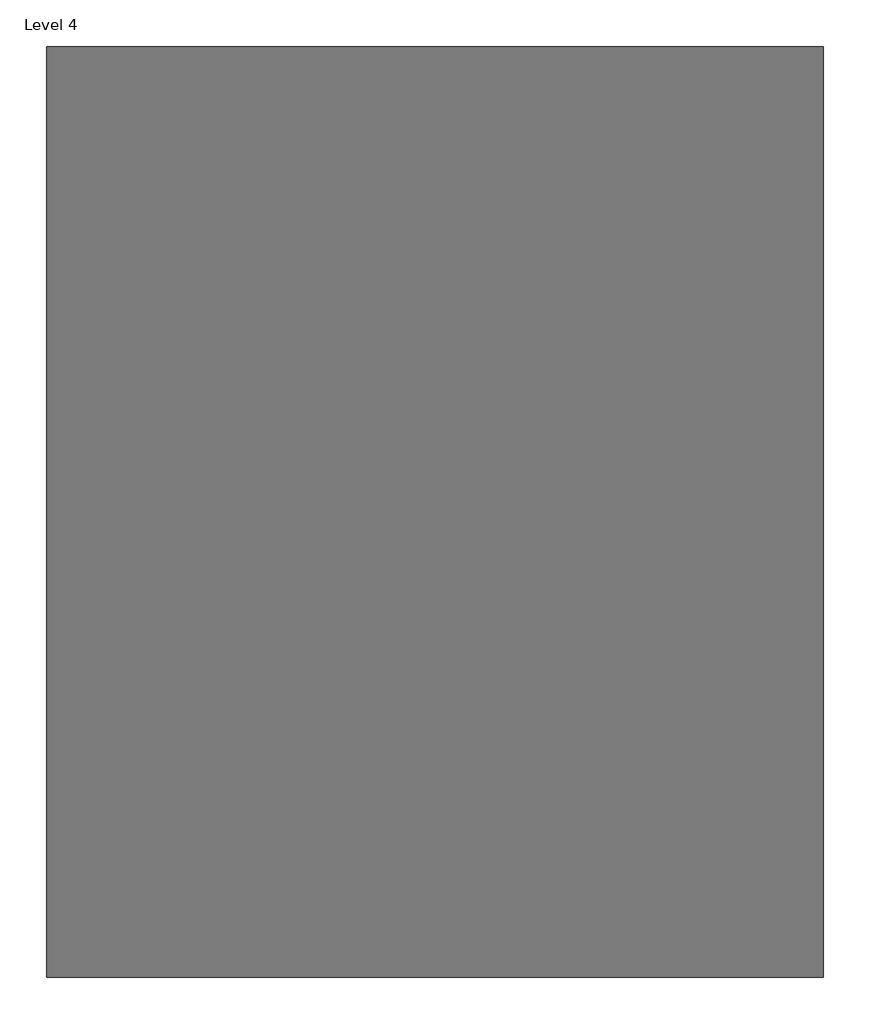
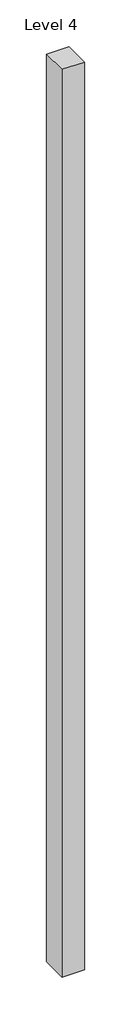
# One storey: 1 proxy.
"""IFC4 building model written with IfcOpenShell, lengths in millimetres."""

from ifc_helpers import new_model, si_unit, origin, place, context, project, spatial, transform, mapped, element, save
from components import generic_models_4_generic_models_4_de7c2597

model = new_model("IFC4")

# Units and contexts
model_context = context("Model", 3, world=origin())
ifc_project = project(units=[si_unit("LENGTHUNIT", "METRE", prefix="MILLI")], contexts=[model_context])

# Site, building, storey
site = spatial("IfcSite", under=ifc_project)
building = spatial("IfcBuilding", under=site)
storey = spatial("IfcBuildingStorey", under=building, Name="Level 4", Elevation=6324.6)

# Proxy
placement = place(None, origin())
generic_models_4_generic_models_4_shape = generic_models_4_generic_models_4_de7c2597(model_context)
element("IfcBuildingElementProxy", 1, Name="Generic Models 4 : Generic Models 4", ObjectType="Generic Models 4 : Generic Models 4", at=placement, inside=storey, context=model_context, shape_type="MappedRepresentation", body=[
    mapped(generic_models_4_generic_models_4_shape, transform((0.0, 0.0, 0.0), x_axis=(1.0, 0.0, 0.0), y_axis=(0.0, 1.0, 0.0), z_axis=(0.0, 0.0, 1.0))),
])

save(model, "model.ifc")

# Revit data of these elements
# Element 1 (IfcBuildingElementProxy, "Generic Models 4 : Generic Models 4")
#   Phase Created = New Construction
